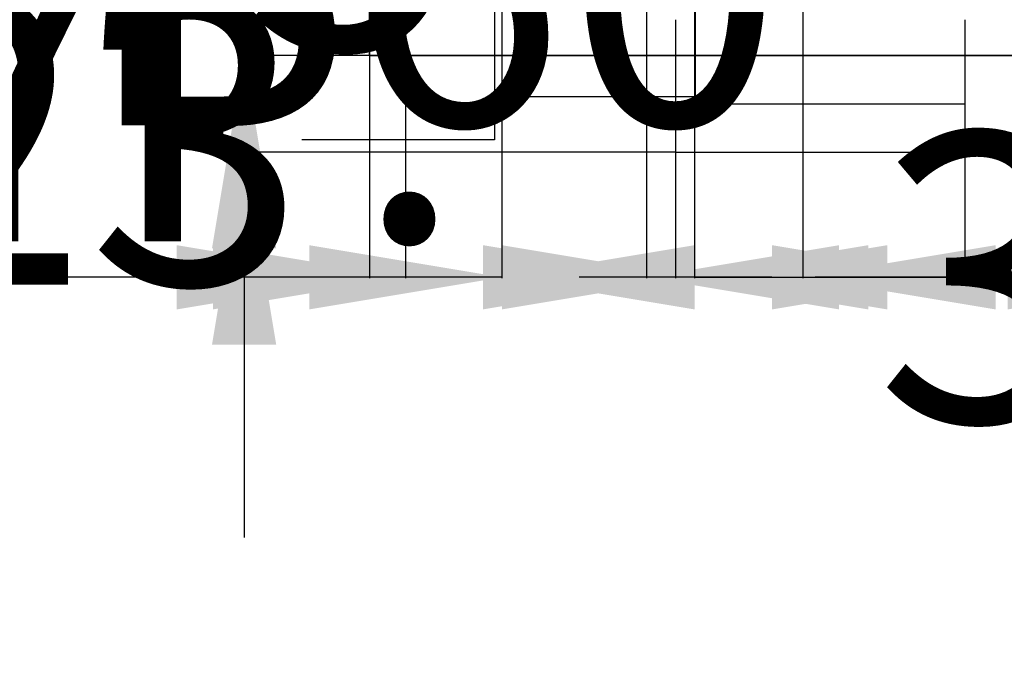
# Model space of a CAD drawing. Units: inches. Extents: x -307 to 2141, y -58 to 895.
# Tile 3 of 28: x 469 to 714, y -58 to 100. Entities that reach past the tile are written whole.
import ezdxf

# ---------------------------------------------------------------- set-up
doc = ezdxf.new("R2010")
doc.units = ezdxf.units.IN
doc.header["$MEASUREMENT"] = 0
for name, color, linetype, lineweight in [('A-ANNO-DIMS', 2, 'Continuous', 18), ('A-FLOR-STRS', 7, 'Continuous', 25), ('A-WALL', 7, 'Continuous', 35)]:
    doc.layers.add(name, color=color, linetype=linetype, lineweight=lineweight)
doc.styles.get("Standard").update_dxf_attribs({"font": 'arial.ttf'})
doc.dimstyles.get("Standard").update_dxf_attribs({"dimtxt": 72, "dimasz": 48, "dimexe": 0.18, "dimexo": 0.0625, "dimgap": 0.09, "dimtad": 0, "dimtih": 1, "dimtoh": 1, "dimdec": 0, "dimrnd": 48, "dimzin": 0, "dimdsep": 46, "dimlunit": 3, "dimtxsty": 'Standard', "dimcen": 0.09, "dimadec": 0, "dimazin": 0, "dimtfac": 1, "dimtdec": 0, "dimtofl": 0, "dimtmove": 0, "dimatfit": 3, "dimfxl": 1, "dimtolj": 1, "dimtzin": 0, "dimarcsym": 0})

# ---------------------------------------------------------------- blocks, each defined once
blk = doc.blocks.new('*D38')
at = {"layer": 'A-ANNO-DIMS', "color": 0, "lineweight": -2, "transparency": 16777216}
for p, q in [((598.5, 222.79), (550.5, 222.79)), ((646.5, 213.85), (646.5, 222.97)), ((706.5, 213.85), (706.5, 222.97)), ((754.5, 222.79), (802.5, 222.79))]:
    blk.add_line(p, q, dxfattribs=at)
at = {"layer": 'A-ANNO-DIMS', "color": 0, "transparency": 16777216}
for points in [[(598.5, 230.79), (598.5, 214.79), (646.5, 222.79)], [(754.5, 230.79), (754.5, 214.79), (706.5, 222.79)]]:
    blk.add_solid(points, dxfattribs=at)
at = {"layer": 'Defpoints', "color": 0, "transparency": 16777216}
for p in [(646.5, 222.79), (646.5, 213.79), (706.5, 213.79)]:
    blk.add_point(p, dxfattribs=at)
at = {"layer": 'A-ANNO-DIMS', "color": 0, "transparency": 16777216, "insert": (97.26, 222.79), "char_height": 72, "attachment_point": 5}
blk.add_mtext('\\A1;LOVESEAT 60 TYP.', dxfattribs=at)
blk = doc.blocks.new('*D39')
at = {"layer": 'A-ANNO-DIMS', "color": 0, "lineweight": -2, "transparency": 16777216}
for p, q in [((637.5, 261.79), (637.5, 309.79)), ((646.43, 213.79), (637.32, 213.79)), ((646.43, 177.12), (637.32, 177.12)), ((637.5, 129.12), (637.5, 81.12)), ((637.5, 81.12), (589.5, 81.12))]:
    blk.add_line(p, q, dxfattribs=at)
at = {"layer": 'A-ANNO-DIMS', "color": 0, "transparency": 16777216}
for points in [[(629.5, 261.79), (645.5, 261.79), (637.5, 213.79)], [(629.5, 129.12), (645.5, 129.12), (637.5, 177.12)]]:
    blk.add_solid(points, dxfattribs=at)
at = {"layer": 'Defpoints', "color": 0, "transparency": 16777216}
for p in [(646.5, 213.79), (637.5, 177.12), (646.5, 177.12)]:
    blk.add_point(p, dxfattribs=at)
at = {"layer": 'A-ANNO-DIMS', "color": 0, "transparency": 16777216, "insert": (414.2, 81.12), "char_height": 72, "attachment_point": 5}
blk.add_mtext('\\A1;37 TYP.', dxfattribs=at)
blk = doc.blocks.new('*D40')
at = {"layer": 'A-ANNO-DIMS', "color": 0, "lineweight": -2, "transparency": 16777216}
for p, q in [((725.38, 128.89), (725.38, 123.17)), ((762.77, 128.89), (762.77, 123.17)), ((677.38, 123.35), (629.38, 123.35)), ((810.77, 123.35), (858.77, 123.35))]:
    blk.add_line(p, q, dxfattribs=at)
at = {"layer": 'A-ANNO-DIMS', "color": 0, "transparency": 16777216}
for points in [[(677.38, 131.35), (677.38, 115.35), (725.38, 123.35)], [(810.77, 131.35), (810.77, 115.35), (762.77, 123.35)]]:
    blk.add_solid(points, dxfattribs=at)
at = {"layer": 'Defpoints', "color": 0, "transparency": 16777216}
for p in [(725.38, 128.96), (762.77, 128.96), (762.77, 123.35)]:
    blk.add_point(p, dxfattribs=at)
at = {"layer": 'A-ANNO-DIMS', "color": 0, "transparency": 16777216, "insert": (1208.37, 123.35), "char_height": 72, "attachment_point": 5}
blk.add_mtext('\\A1;PLANT 37 TYP.', dxfattribs=at)
blk = doc.blocks.new('*D48')
at = {"layer": 'A-ANNO-DIMS', "color": 0, "lineweight": -2, "transparency": 16777216}
for p, q in [((724, 313.98), (724, 361.98)), ((732.94, 265.98), (723.82, 265.98)), ((732.94, 205.98), (723.82, 205.98)), ((724, 157.98), (724, 109.98)), ((724, 109.98), (676, 109.98))]:
    blk.add_line(p, q, dxfattribs=at)
at = {"layer": 'A-ANNO-DIMS', "color": 0, "transparency": 16777216}
for points in [[(716, 313.98), (732, 313.98), (724, 265.98)], [(716, 157.98), (732, 157.98), (724, 205.98)]]:
    blk.add_solid(points, dxfattribs=at)
at = {"layer": 'Defpoints', "color": 0, "transparency": 16777216}
for p in [(733, 265.98), (724, 205.98), (733, 205.98)]:
    blk.add_point(p, dxfattribs=at)
at = {"layer": 'A-ANNO-DIMS', "color": 0, "transparency": 16777216, "insert": (321.56, 109.98), "char_height": 72, "attachment_point": 5}
blk.add_mtext('\\A1;MEDIA UNIT 60', dxfattribs=at)
blk = doc.blocks.new('*D63')
at = {"layer": 'A-ANNO-DIMS', "color": 0, "lineweight": -2, "transparency": 16777216}
for p, q in [((916.4, 691.34), (947.72, 691.34)), ((947.54, 643.34), (947.54, 416.19)), ((947.54, 115.34), (947.54, 342.49)), ((704.68, 67.34), (947.72, 67.34))]:
    blk.add_line(p, q, dxfattribs=at)
at = {"layer": 'A-ANNO-DIMS', "color": 0, "transparency": 16777216}
for points in [[(939.54, 643.34), (955.54, 643.34), (947.54, 691.34)], [(939.54, 115.34), (955.54, 115.34), (947.54, 67.34)]]:
    blk.add_solid(points, dxfattribs=at)
at = {"layer": 'Defpoints', "color": 0, "transparency": 16777216}
for p in [(916.34, 691.34), (704.62, 67.34), (947.54, 67.34)]:
    blk.add_point(p, dxfattribs=at)
at = {"layer": 'A-ANNO-DIMS', "color": 0, "transparency": 16777216, "insert": (947.54, 379.34), "char_height": 72, "attachment_point": 5}
blk.add_mtext('\\A1;624', dxfattribs=at)
blk = doc.blocks.new('*D65')
at = {"layer": 'A-ANNO-DIMS', "color": 0, "lineweight": -2, "transparency": 16777216}
for p, q in [((587.54, 252.57), (587.54, 300.57)), ((556.4, 204.57), (587.72, 204.57)), ((556.4, 166.34), (587.72, 166.34)), ((587.54, 118.34), (587.54, 70.34)), ((587.54, 70.34), (539.54, 70.34))]:
    blk.add_line(p, q, dxfattribs=at)
at = {"layer": 'A-ANNO-DIMS', "color": 0, "transparency": 16777216}
for points in [[(579.54, 252.57), (595.54, 252.57), (587.54, 204.57)], [(579.54, 118.34), (595.54, 118.34), (587.54, 166.34)]]:
    blk.add_solid(points, dxfattribs=at)
at = {"layer": 'Defpoints', "color": 0, "transparency": 16777216}
for p in [(556.34, 204.57), (556.34, 166.34), (587.54, 166.34)]:
    blk.add_point(p, dxfattribs=at)
at = {"layer": 'A-ANNO-DIMS', "color": 0, "transparency": 16777216, "insert": (417.99, 70.34), "char_height": 72, "attachment_point": 5}
blk.add_mtext('\\A1;38.23', dxfattribs=at)
blk = doc.blocks.new('*D70')
at = {"layer": 'A-ANNO-DIMS', "color": 0, "lineweight": -2, "transparency": 16777216}
for p, q in [((525.13184, 214.340828), (525.13184, 262.340828)), ((556.27334, 166.340828), (524.95184, 166.340828)), ((556.27334, 91.340828), (524.95184, 91.340828)), ((525.13184, 43.340828), (525.13184, -4.659172))]:
    blk.add_line(p, q, dxfattribs=at)
at = {"layer": 'A-ANNO-DIMS', "color": 0, "transparency": 16777216}
for points in [[(517.13184, 214.340828), (533.13184, 214.340828), (525.13184, 166.340828)], [(517.13184, 43.340828), (533.13184, 43.340828), (525.13184, 91.340828)]]:
    blk.add_solid(points, dxfattribs=at)
at = {"layer": 'Defpoints', "color": 0, "transparency": 16777216}
for p in [(525.13184, 166.340828), (556.33584, 166.340828), (556.33584, 91.340828)]:
    blk.add_point(p, dxfattribs=at)
at = {"layer": 'A-ANNO-DIMS', "color": 0, "transparency": 16777216, "insert": (525.13184, 128.840828), "char_height": 72, "attachment_point": 5}
blk.add_mtext('\\A1;75', dxfattribs=at)
blk = doc.blocks.new('*D71')
at = {"layer": 'A-ANNO-DIMS', "color": 0, "lineweight": -2, "transparency": 16777216}
for p, q in [((525.13, 139.34), (525.13, 187.34)), ((525.13, 187.34), (573.13, 187.34)), ((632.56, 91.34), (524.95, 91.34)), ((632.56, 67.34), (524.95, 67.34)), ((525.13, 19.34), (525.13, -28.66))]:
    blk.add_line(p, q, dxfattribs=at)
at = {"layer": 'A-ANNO-DIMS', "color": 0, "transparency": 16777216}
for points in [[(517.13, 139.34), (533.13, 139.34), (525.13, 91.34)], [(517.13, 19.34), (533.13, 19.34), (525.13, 67.34)]]:
    blk.add_solid(points, dxfattribs=at)
at = {"layer": 'Defpoints', "color": 0, "transparency": 16777216}
for p in [(525.13, 91.34), (632.62, 91.34), (632.62, 67.34)]:
    blk.add_point(p, dxfattribs=at)
at = {"layer": 'A-ANNO-DIMS', "color": 0, "transparency": 16777216, "insert": (625.26, 187.34), "char_height": 72, "attachment_point": 5}
blk.add_mtext('\\A1;24', dxfattribs=at)
blk = doc.blocks.new('*D72')
at = {"layer": 'A-ANNO-DIMS', "color": 0, "lineweight": -2, "transparency": 16777216}
for p, q in [((556.34, 91.28), (556.34, 35.96)), ((632.62, 91.28), (632.62, 35.96)), ((508.34, 36.14), (460.34, 36.14)), ((680.62, 36.14), (728.62, 36.14))]:
    blk.add_line(p, q, dxfattribs=at)
at = {"layer": 'A-ANNO-DIMS', "color": 0, "transparency": 16777216}
for points in [[(508.34, 44.14), (508.34, 28.14), (556.34, 36.14)], [(680.62, 44.14), (680.62, 28.14), (632.62, 36.14)]]:
    blk.add_solid(points, dxfattribs=at)
at = {"layer": 'Defpoints', "color": 0, "transparency": 16777216}
for p in [(556.34, 91.34), (632.62, 91.34), (632.62, 36.14)]:
    blk.add_point(p, dxfattribs=at)
at = {"layer": 'A-ANNO-DIMS', "color": 0, "transparency": 16777216, "insert": (849.97, 36.14), "char_height": 72, "attachment_point": 5}
blk.add_mtext('\\A1;76.29', dxfattribs=at)
blk = doc.blocks.new('*D73')
at = {"layer": 'A-ANNO-DIMS', "color": 0, "lineweight": -2, "transparency": 16777216}
for p, q in [((632.62, 91.28), (632.62, 35.96)), ((704.62, 91.28), (704.62, 35.96)), ((584.62, 36.14), (536.62, 36.14)), ((752.62, 36.14), (800.62, 36.14))]:
    blk.add_line(p, q, dxfattribs=at)
at = {"layer": 'A-ANNO-DIMS', "color": 0, "transparency": 16777216}
for points in [[(584.62, 44.14), (584.62, 28.14), (632.62, 36.14)], [(752.62, 44.14), (752.62, 28.14), (704.62, 36.14)]]:
    blk.add_solid(points, dxfattribs=at)
at = {"layer": 'Defpoints', "color": 0, "transparency": 16777216}
for p in [(632.62, 91.34), (704.62, 91.34), (704.62, 36.14)]:
    blk.add_point(p, dxfattribs=at)
at = {"layer": 'A-ANNO-DIMS', "color": 0, "transparency": 16777216, "insert": (851.62, 36.14), "char_height": 72, "attachment_point": 5}
blk.add_mtext('\\A1;72', dxfattribs=at)
blk = doc.blocks.new('*D74')
at = {"layer": 'A-ANNO-DIMS', "color": 0, "lineweight": -2, "transparency": 16777216}
for p, q in [((704.62, 91.28), (704.62, 35.96)), ((772.34, 91.28), (772.34, 35.96)), ((656.62, 36.14), (608.62, 36.14)), ((820.34, 36.14), (868.34, 36.14))]:
    blk.add_line(p, q, dxfattribs=at)
at = {"layer": 'A-ANNO-DIMS', "color": 0, "transparency": 16777216}
for points in [[(656.62, 44.14), (656.62, 28.14), (704.62, 36.14)], [(820.34, 44.14), (820.34, 28.14), (772.34, 36.14)]]:
    blk.add_solid(points, dxfattribs=at)
at = {"layer": 'Defpoints', "color": 0, "transparency": 16777216}
for p in [(704.62, 91.34), (772.34, 91.34), (772.34, 36.14)]:
    blk.add_point(p, dxfattribs=at)
at = {"layer": 'A-ANNO-DIMS', "color": 0, "transparency": 16777216, "insert": (983.15, 36.14), "char_height": 72, "attachment_point": 5}
blk.add_mtext('\\A1;67.71', dxfattribs=at)
blk = doc.blocks.new('*D86')
at = {"layer": 'A-ANNO-DIMS', "color": 0, "lineweight": -2, "transparency": 16777216}
for p, q in [((565.34, 304.28), (565.34, 35.96)), ((625.34, 304.28), (625.34, 35.96)), ((517.34, 36.14), (469.34, 36.14)), ((673.34, 36.14), (721.34, 36.14))]:
    blk.add_line(p, q, dxfattribs=at)
at = {"layer": 'A-ANNO-DIMS', "color": 0, "transparency": 16777216}
for points in [[(517.34, 44.14), (517.34, 28.14), (565.34, 36.14)], [(673.34, 44.14), (673.34, 28.14), (625.34, 36.14)]]:
    blk.add_solid(points, dxfattribs=at)
at = {"layer": 'Defpoints', "color": 0, "transparency": 16777216}
for p in [(565.34, 304.34), (625.34, 304.34), (625.34, 36.14)]:
    blk.add_point(p, dxfattribs=at)
at = {"layer": 'A-ANNO-DIMS', "color": 0, "transparency": 16777216, "insert": (773.07, 36.14), "char_height": 72, "attachment_point": 5}
blk.add_mtext('\\A1;60', dxfattribs=at)
blk = doc.blocks.new('*D90')
at = {"layer": 'A-ANNO-DIMS', "color": 0, "lineweight": -2, "transparency": 16777216}
for p, q in [((556.34, 166.28), (556.34, 35.96)), ((589.34, 166.28), (589.34, 35.96)), ((508.34, 36.14), (460.34, 36.14)), ((637.34, 36.14), (685.34, 36.14))]:
    blk.add_line(p, q, dxfattribs=at)
at = {"layer": 'A-ANNO-DIMS', "color": 0, "transparency": 16777216}
for points in [[(508.34, 44.14), (508.34, 28.14), (556.34, 36.14)], [(637.34, 44.14), (637.34, 28.14), (589.34, 36.14)]]:
    blk.add_solid(points, dxfattribs=at)
at = {"layer": 'Defpoints', "color": 0, "transparency": 16777216}
for p in [(556.34, 166.34), (589.34, 166.34), (589.34, 36.14)]:
    blk.add_point(p, dxfattribs=at)
at = {"layer": 'A-ANNO-DIMS', "color": 0, "transparency": 16777216, "insert": (736.97, 36.14), "char_height": 72, "attachment_point": 5}
blk.add_mtext('\\A1;33', dxfattribs=at)
blk = doc.blocks.new('*D91')
at = {"layer": 'A-ANNO-DIMS', "color": 0, "lineweight": -2, "transparency": 16777216}
for p, q in [((589.34, 166.28), (589.34, 35.96)), ((637.34, 166.28), (637.34, 35.96)), ((541.34, 36.14), (493.34, 36.14)), ((685.34, 36.14), (733.34, 36.14))]:
    blk.add_line(p, q, dxfattribs=at)
at = {"layer": 'A-ANNO-DIMS', "color": 0, "transparency": 16777216}
for points in [[(541.34, 44.14), (541.34, 28.14), (589.34, 36.14)], [(685.34, 44.14), (685.34, 28.14), (637.34, 36.14)]]:
    blk.add_solid(points, dxfattribs=at)
at = {"layer": 'Defpoints', "color": 0, "transparency": 16777216}
for p in [(589.34, 166.34), (637.34, 166.34), (637.34, 36.14)]:
    blk.add_point(p, dxfattribs=at)
at = {"layer": 'A-ANNO-DIMS', "color": 0, "transparency": 16777216, "insert": (786.52, 36.14), "char_height": 72, "attachment_point": 5}
blk.add_mtext('\\A1;48', dxfattribs=at)
blk = doc.blocks.new('*D92')
at = {"layer": 'A-ANNO-DIMS', "color": 0, "lineweight": -2, "transparency": 16777216}
for p, q in [((637.34, 166.28), (637.34, 35.96)), ((664.34, 166.28), (664.34, 35.96)), ((589.34, 36.14), (541.34, 36.14)), ((712.34, 36.14), (760.34, 36.14))]:
    blk.add_line(p, q, dxfattribs=at)
at = {"layer": 'A-ANNO-DIMS', "color": 0, "transparency": 16777216}
for points in [[(589.34, 44.14), (589.34, 28.14), (637.34, 36.14)], [(712.34, 44.14), (712.34, 28.14), (664.34, 36.14)]]:
    blk.add_solid(points, dxfattribs=at)
at = {"layer": 'Defpoints', "color": 0, "transparency": 16777216}
for p in [(637.34, 166.34), (664.34, 166.34), (664.34, 36.14)]:
    blk.add_point(p, dxfattribs=at)
at = {"layer": 'A-ANNO-DIMS', "color": 0, "transparency": 16777216, "insert": (812.61, 36.14), "char_height": 72, "attachment_point": 5}
blk.add_mtext('\\A1;27', dxfattribs=at)
blk = doc.blocks.new('*D99')
at = {"layer": 'A-ANNO-DIMS', "color": 0, "lineweight": -2, "transparency": 16777216}
for p, q in [((763.34, 481.28), (763.34, 35.96)), ((802.34, 481.28), (802.34, 35.96)), ((715.34, 36.14), (667.34, 36.14)), ((850.34, 36.14), (898.34, 36.14))]:
    blk.add_line(p, q, dxfattribs=at)
at = {"layer": 'A-ANNO-DIMS', "color": 0, "transparency": 16777216}
for points in [[(715.34, 44.14), (715.34, 28.14), (763.34, 36.14)], [(850.34, 44.14), (850.34, 28.14), (802.34, 36.14)]]:
    blk.add_solid(points, dxfattribs=at)
at = {"layer": 'Defpoints', "color": 0, "transparency": 16777216}
for p in [(763.34, 481.34), (802.34, 481.34), (802.34, 36.14)]:
    blk.add_point(p, dxfattribs=at)
at = {"layer": 'A-ANNO-DIMS', "color": 0, "transparency": 16777216, "insert": (950.04, 36.14), "char_height": 72, "attachment_point": 5}
blk.add_mtext('\\A1;39', dxfattribs=at)
blk = doc.blocks.new('*D100')
at = {"layer": 'A-ANNO-DIMS', "color": 0, "lineweight": -2, "transparency": 16777216}
for p, q in [((589.34, 409.28), (589.34, 35.96)), ((625.34, 409.28), (625.34, 35.96)), ((541.34, 36.14), (493.34, 36.14)), ((673.34, 36.14), (721.34, 36.14))]:
    blk.add_line(p, q, dxfattribs=at)
at = {"layer": 'A-ANNO-DIMS', "color": 0, "transparency": 16777216}
for points in [[(541.34, 44.14), (541.34, 28.14), (589.34, 36.14)], [(673.34, 44.14), (673.34, 28.14), (625.34, 36.14)]]:
    blk.add_solid(points, dxfattribs=at)
at = {"layer": 'Defpoints', "color": 0, "transparency": 16777216}
for p in [(589.34, 409.34), (625.34, 409.34), (625.34, 36.14)]:
    blk.add_point(p, dxfattribs=at)
at = {"layer": 'A-ANNO-DIMS', "color": 0, "transparency": 16777216, "insert": (772.95, 36.14), "char_height": 72, "attachment_point": 5}
blk.add_mtext('\\A1;36', dxfattribs=at)

msp = doc.modelspace()

# ---------------------------------------------------------------- linework, layer by layer
at = {"layer": 'A-FLOR-STRS'}
for p, q in [((632.6211, 100.2545), (632.6211, 91.3408)), ((704.6211, 100.2545), (704.6211, 91.3408)), ((632.6211, 91.3408), (632.6211, 79.3408)), ((704.6211, 91.3408), (704.6211, 79.3408)), ((632.6211, 79.3408), (704.6211, 79.3408)), ((632.6211, 79.3408), (704.6211, 79.3408)), ((632.6211, 79.3408), (632.6211, 67.3408)), ((704.6211, 79.3408), (704.6211, 67.3408)), ((632.6211, 67.3408), (704.6211, 67.3408))]:
    msp.add_line(p, q, dxfattribs=at)
at = {"layer": 'A-WALL'}
for p, q in [((556.3358, 691.3408), (556.3358, 91.3408)), ((556.3358, 91.3408), (772.3358, 91.3408))]:
    msp.add_line(p, q, dxfattribs=at)

# ---------------------------------------------------------------- dimensions: what is measured, and where the dimension line sits
at = {"layer": 'A-ANNO-DIMS'}
for base, p1, p2, angle, override, picture, middle in [((947.5398, 67.3408), (916.3358, 691.3408), (704.6211, 67.3408), 90, {"dimdec": 0, "dimlfac": 1, "dimrnd": 0, "dimzin": 0, "dimdsep": 46, "dimlunit": 2}, '*D63', (947.5398, 379.3408)), ((587.5398, 166.3408), (556.3358, 204.574), (556.3358, 166.3408), 270, {"dimdec": 2, "dimlfac": 1, "dimrnd": 0, "dimzin": 0, "dimdsep": 46, "dimlunit": 2}, '*D65', (417.9928, 70.3408)), ((525.1318, 166.3408), (556.3358, 91.3408), (556.3358, 166.3408), 90, {"dimdec": 0, "dimlfac": 1, "dimrnd": 0, "dimzin": 0, "dimdsep": 46, "dimlunit": 2}, '*D70', (525.1318, 128.8408)), ((525.1318, 91.3408), (632.6211, 67.3408), (632.6211, 91.3408), 90, {"dimdec": 0, "dimlfac": 1, "dimrnd": 0, "dimzin": 0, "dimdsep": 46, "dimlunit": 2}, '*D71', (625.2573, 187.3408))]:
    dim = msp.add_linear_dim(base=base, p1=p1, p2=p2, angle=angle, dimstyle='Standard', override=override, dxfattribs=at)
    dim.commit()
    dim.dimension.update_dxf_attribs({"geometry": picture, "text_midpoint": middle})
for base, p1, p2, override, picture, middle in [((802.3358, 36.1368), (763.3358, 481.3408), (802.3358, 481.3408), {"dimdec": 0, "dimlfac": 1, "dimrnd": 0, "dimzin": 0, "dimdsep": 46, "dimlunit": 2}, '*D99', (950.0438, 36.1368)), ((625.3358, 36.1368), (589.339, 409.3408), (625.3358, 409.3408), {"dimdec": 0, "dimlfac": 1, "dimrnd": 0, "dimzin": 0, "dimdsep": 46, "dimlunit": 2}, '*D100', (772.9456, 36.1368)), ((625.3358, 36.1368), (565.3358, 304.3408), (625.3358, 304.3408), {"dimdec": 0, "dimlfac": 1, "dimrnd": 0, "dimzin": 0, "dimdsep": 46, "dimlunit": 2}, '*D86', (773.0684, 36.1368)), ((589.3358, 36.1368), (556.3358, 166.3408), (589.3358, 166.3408), {"dimdec": 0, "dimlfac": 1, "dimrnd": 0, "dimzin": 0, "dimdsep": 46, "dimlunit": 2}, '*D90', (736.9702, 36.1368)), ((637.3358, 36.1368), (589.3358, 166.3408), (637.3358, 166.3408), {"dimdec": 0, "dimlfac": 1, "dimrnd": 0, "dimzin": 0, "dimdsep": 46, "dimlunit": 2}, '*D91', (786.5172, 36.1368)), ((664.3358, 36.1368), (637.3358, 166.3408), (664.3358, 166.3408), {"dimdec": 0, "dimlfac": 1, "dimrnd": 0, "dimzin": 0, "dimdsep": 46, "dimlunit": 2}, '*D92', (812.6087, 36.1368)), ((632.6211, 36.1368), (556.3358, 91.3408), (632.6211, 91.3408), {"dimdec": 2, "dimlfac": 1, "dimrnd": 0, "dimzin": 0, "dimdsep": 46, "dimlunit": 2}, '*D72', (849.9716, 36.1368)), ((704.6211, 36.1368), (632.6211, 91.3408), (704.6211, 91.3408), {"dimdec": 0, "dimlfac": 1, "dimrnd": 0, "dimzin": 0, "dimdsep": 46, "dimlunit": 2}, '*D73', (851.6169, 36.1368)), ((772.3358, 36.1368), (704.6211, 91.3408), (772.3358, 91.3408), {"dimdec": 2, "dimlfac": 1, "dimrnd": 0, "dimzin": 0, "dimdsep": 46, "dimlunit": 2}, '*D74', (983.1544, 36.1368))]:
    dim = msp.add_linear_dim(base=base, p1=p1, p2=p2, dimstyle='Standard', override=override, dxfattribs=at)
    dim.commit()
    dim.dimension.update_dxf_attribs({"geometry": picture, "text_midpoint": middle})
for base, p1, p2, angle, text, picture, middle in [((646.4965, 222.7908), (706.4965, 213.7908), (646.4965, 213.7908), 180, 'LOVESEAT <> TYP.', '*D38', (97.2632, 222.7908)), ((724.0025, 205.9815), (733.0025, 265.9815), (733.0025, 205.9815), 270, 'MEDIA UNIT <>', '*D48', (321.5605, 109.9815)), ((637.4965, 177.1242), (646.4965, 213.7908), (646.4965, 177.1242), 270, '<> TYP.', '*D39', (414.195, 81.1242))]:
    dim = msp.add_linear_dim(base=base, p1=p1, p2=p2, angle=angle, text=text, dimstyle='Standard', override={"dimdec": 0, "dimlfac": 1, "dimrnd": 0, "dimzin": 0, "dimdsep": 46, "dimlunit": 2}, dxfattribs=at)
    dim.commit()
    dim.dimension.update_dxf_attribs({"geometry": picture, "text_midpoint": middle})
dim = msp.add_linear_dim(base=(762.7703, 123.348), p1=(725.3775, 128.9569), p2=(762.7703, 128.9569), text='PLANT <> TYP.', dimstyle='Standard', override={"dimdec": 0, "dimlfac": 1, "dimrnd": 0, "dimzin": 0, "dimdsep": 46, "dimlunit": 2}, dxfattribs=at)
dim.commit()
dim.dimension.update_dxf_attribs({"geometry": '*D40', "text_midpoint": (1208.3746, 123.348)})

doc.saveas('drawing.dxf')
